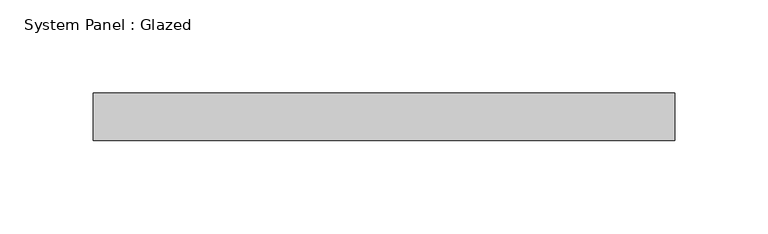
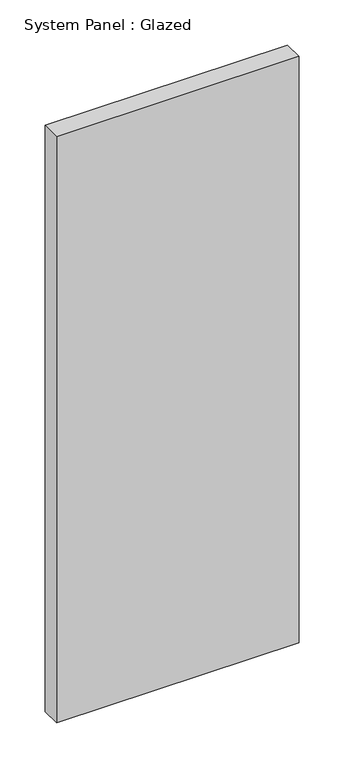
"""IFC4 building model written with IfcOpenShell, lengths in millimetres: plate geometry, System Panel : Glazed."""

from ifc_helpers import new_model, si_unit, origin, origin_with_axes, place, context, project, spatial, polyline, outline, extrude, source, transform, mapped, element, save


def system_panel_glazed_1557c927(model_context):
    return source(origin(), model_context, "Body", "SweptSolid", [
        extrude(outline(polyline([(155.575, 19.05), (-155.575, 19.05), (-155.575, 44.45), (155.575, 44.45), (155.575, 19.05)])), origin_with_axes(), (0.0, 0.0, 1.0), 793.75),
    ])


if __name__ == "__main__":
    model = new_model("IFC4")
    model_context = context("Model", 3, world=origin())
    ifc_project = project(units=[si_unit("LENGTHUNIT", "METRE", prefix="MILLI")], contexts=[model_context])
    site = spatial("IfcSite", under=ifc_project)
    building = spatial("IfcBuilding", under=site)
    placement = place(None, origin())
    system_panel_glazed_shape = system_panel_glazed_1557c927(model_context)
    element("IfcPlate", 1, ObjectType="System Panel : Glazed", at=placement, inside=building, context=model_context, shape_type="MappedRepresentation", body=[
        mapped(system_panel_glazed_shape, transform((0.0, 0.0, 0.0), x_axis=(1.0, 0.0, 0.0), y_axis=(0.0, 1.0, 0.0), z_axis=(0.0, 0.0, 1.0))),
    ])
    save(model, "model.ifc")

# Revit data of these elements
# Type "System Panel : Glazed"
#   Construction Type Id = "GSP4R"
#   Analytic Construction = "1/8 in Pilkington single glazing"
#   Visual Light Transmittance = 0.9
#   Solar Heat Gain Coefficient = 0.86
#   Heat Transfer Coefficient (U) = 1.18115 BTU/(h·ft²·°F)
# Element 1 (IfcPlate, "System Panel : Glazed")
#   Materials on its faces: "Glass"
# Materials
#   "Glass": class "Glass", colour RGB 0 128 192, transparency 0.75, Description = "Soda Lime Glass", Cost = 0
